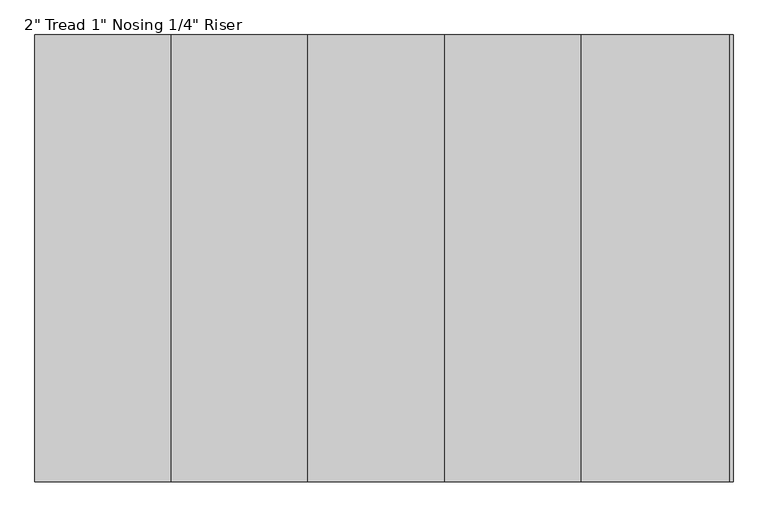
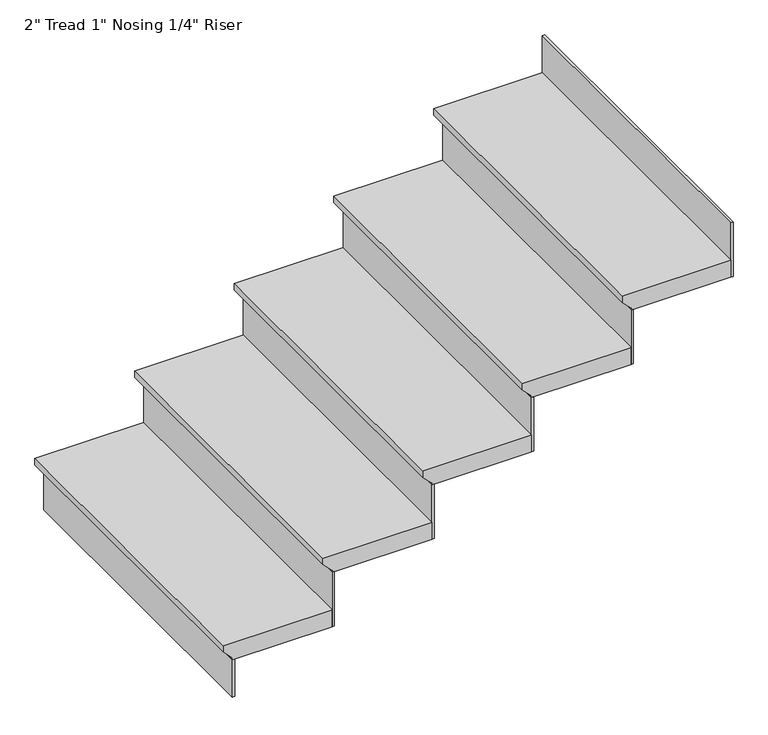
"""IFC4 building model written with IfcOpenShell, lengths in millimetres: stair flight geometry."""

from ifc_helpers import new_model, si_unit, frame, origin, place, context, project, spatial, polyline, outline, extrude, source, transform, mapped, element, save


def stair_flight_7b3f2189(model_context):
    return source(origin(), model_context, "Body", "SweptSolid", [
        extrude(outline(polyline([(466.1647059, 1603.1430349), (466.1647059, 1298.3430349), (447.1147059, 1298.3430349), (421.7147059, 1323.7430349), (415.3647059, 1323.7430349), (415.3647059, 1603.1430349), (466.1647059, 1603.1430349)])), frame((0.0, 4166.2555142, 0.0), z_axis=(0.0, 1.0, 0.0), x_axis=(0.0, 0.0, 1.0)), (0.0, 0.0, 1.0), 914.4),
        extrude(outline(polyline([(1330.0930349, 4166.2555142), (1323.7430349, 4166.2555142), (1323.7430349, 5080.6555142), (1330.0930349, 5080.6555142), (1330.0930349, 4166.2555142)])), frame((0.0, 0.0, 304.8), z_axis=(0.0, 0.0, 1.0), x_axis=(1.0, 0.0, 0.0)), (0.0, 0.0, 1.0), 110.5647059),
        extrude(outline(polyline([(1609.4930349, 4166.2555142), (1603.1430349, 4166.2555142), (1603.1430349, 5080.6555142), (1609.4930349, 5080.6555142), (1609.4930349, 4166.2555142)])), frame((0.0, 0.0, 415.3647059), z_axis=(0.0, 0.0, 1.0), x_axis=(1.0, 0.0, 0.0)), (0.0, 0.0, 1.0), 161.3647059),
        extrude(outline(polyline([(627.5294118, 1882.5430349), (627.5294118, 1577.7430349), (608.4794118, 1577.7430349), (583.0794118, 1603.1430349), (576.7294118, 1603.1430349), (576.7294118, 1882.5430349), (627.5294118, 1882.5430349)])), frame((0.0, 4166.2555142, 0.0), z_axis=(0.0, 1.0, 0.0), x_axis=(0.0, 0.0, 1.0)), (0.0, 0.0, 1.0), 914.4),
        extrude(outline(polyline([(1888.8930349, 4166.2555142), (1882.5430349, 4166.2555142), (1882.5430349, 5080.6555142), (1888.8930349, 5080.6555142), (1888.8930349, 4166.2555142)])), frame((0.0, 0.0, 576.7294118), z_axis=(0.0, 0.0, 1.0), x_axis=(1.0, 0.0, 0.0)), (0.0, 0.0, 1.0), 161.3647059),
        extrude(outline(polyline([(788.8941176, 2161.9430349), (788.8941176, 1857.1430349), (769.8441176, 1857.1430349), (744.4441176, 1882.5430349), (738.0941176, 1882.5430349), (738.0941176, 2161.9430349), (788.8941176, 2161.9430349)])), frame((0.0, 4166.2555142, 0.0), z_axis=(0.0, 1.0, 0.0), x_axis=(0.0, 0.0, 1.0)), (0.0, 0.0, 1.0), 914.4),
        extrude(outline(polyline([(2168.2930349, 4166.2555142), (2161.9430349, 4166.2555142), (2161.9430349, 5080.6555142), (2168.2930349, 5080.6555142), (2168.2930349, 4166.2555142)])), frame((0.0, 0.0, 738.0941176), z_axis=(0.0, 0.0, 1.0), x_axis=(1.0, 0.0, 0.0)), (0.0, 0.0, 1.0), 161.3647059),
        extrude(outline(polyline([(950.2588235, 2441.3430349), (950.2588235, 2136.5430349), (931.2088235, 2136.5430349), (905.8088235, 2161.9430349), (899.4588235, 2161.9430349), (899.4588235, 2441.3430349), (950.2588235, 2441.3430349)])), frame((0.0, 4166.2555142, 0.0), z_axis=(0.0, 1.0, 0.0), x_axis=(0.0, 0.0, 1.0)), (0.0, 0.0, 1.0), 914.4),
        extrude(outline(polyline([(2447.6930349, 4166.2555142), (2441.3430349, 4166.2555142), (2441.3430349, 5080.6555142), (2447.6930349, 5080.6555142), (2447.6930349, 4166.2555142)])), frame((0.0, 0.0, 899.4588235), z_axis=(0.0, 0.0, 1.0), x_axis=(1.0, 0.0, 0.0)), (0.0, 0.0, 1.0), 161.3647059),
        extrude(outline(polyline([(1111.6235294, 2720.7430349), (1111.6235294, 2415.9430349), (1092.5735294, 2415.9430349), (1067.1735294, 2441.3430349), (1060.8235294, 2441.3430349), (1060.8235294, 2720.7430349), (1111.6235294, 2720.7430349)])), frame((0.0, 4166.2555142, 0.0), z_axis=(0.0, 1.0, 0.0), x_axis=(0.0, 0.0, 1.0)), (0.0, 0.0, 1.0), 914.4),
        extrude(outline(polyline([(2727.0930349, 4166.2555142), (2720.7430349, 4166.2555142), (2720.7430349, 5080.6555142), (2727.0930349, 5080.6555142), (2727.0930349, 4166.2555142)])), frame((0.0, 0.0, 1060.8235294), z_axis=(0.0, 0.0, 1.0), x_axis=(1.0, 0.0, 0.0)), (0.0, 0.0, 1.0), 161.3647059),
    ])


if __name__ == "__main__":
    model = new_model("IFC4")
    model_context = context("Model", 3, world=origin())
    ifc_project = project(units=[si_unit("LENGTHUNIT", "METRE", prefix="MILLI")], contexts=[model_context])
    site = spatial("IfcSite", under=ifc_project)
    building = spatial("IfcBuilding", under=site)
    placement = place(None, origin())
    stair_flight_shape = stair_flight_7b3f2189(model_context)
    element("IfcStairFlight", 1, ObjectType="2\" Tread 1\" Nosing 1/4\" Riser", at=placement, inside=building, context=model_context, shape_type="MappedRepresentation", body=[
        mapped(stair_flight_shape, transform((0.0, 0.0, 0.0), x_axis=(1.0, 0.0, 0.0), y_axis=(0.0, 1.0, 0.0), z_axis=(0.0, 0.0, 1.0))),
    ])
    save(model, "model.ifc")
